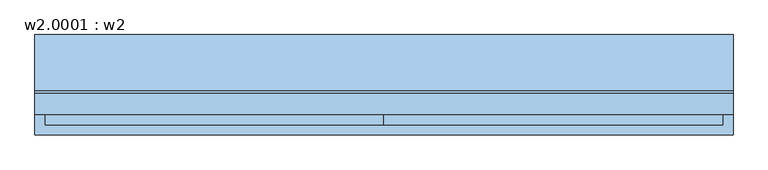
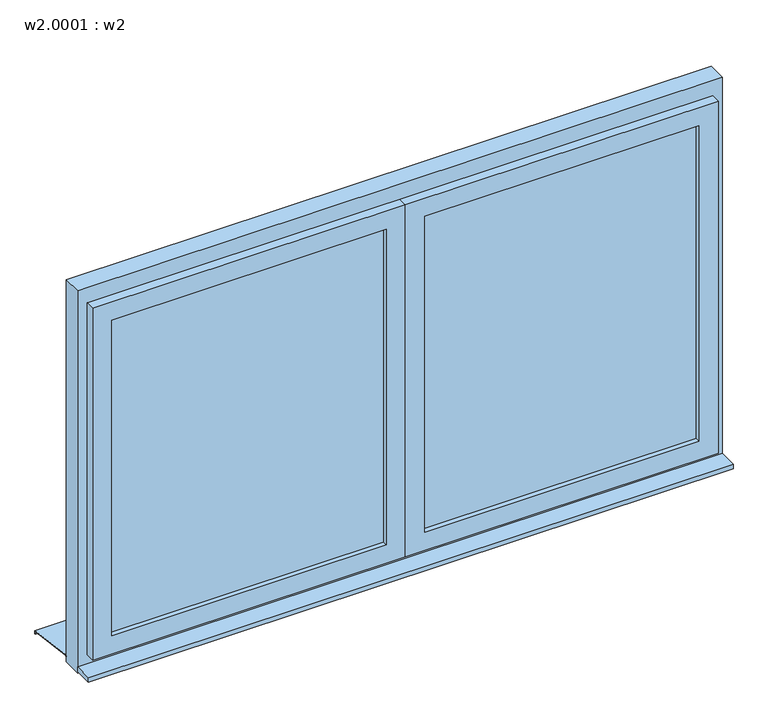
"""IFC4 building model written with IfcOpenShell, lengths in millimetres: window geometry, w2.0001 : w2."""

from ifc_helpers import new_model, si_unit, frame, origin, place, context, project, spatial, polyline, outline, extrude, faceted_brep, source, transform, mapped, element, save


def w2_0001_w2_7b90d420(model_context):
    return source(origin(), model_context, "Body", "SolidModel", [
        extrude(outline(polyline([(-15.6778457, 1020.0), (144.3, 1000.0), (144.3, 990.0), (142.3, 990.0), (142.3, 998.3604634), (-15.8759277, 1018.0), (-25.7, 1018.0), (-25.7, 1020.0), (-15.6778457, 1020.0)])), frame((-1005.0, 0.0, 0.0), z_axis=(1.0, 0.0, 0.0), x_axis=(0.0, 1.0, 0.0)), (0.0, 0.0, 1.0), 2010.0),
        extrude(outline(polyline([(-1005.0, -144.3), (-1005.0, -85.7), (1005.0, -85.7), (1005.0, -144.3), (-1005.0, -144.3)])), frame((0.0, 0.0, 1005.0), z_axis=(0.0, 0.0, 1.0), x_axis=(1.0, 0.0, 0.0)), (0.0, 0.0, 1.0), 15.0),
        extrude(outline(polyline([(60.0, -70.7), (915.0, -70.7), (915.0, -100.7), (60.0, -100.7), (60.0, -70.7)])), frame((0.0, 0.0, 1110.0), z_axis=(0.0, 0.0, 1.0), x_axis=(1.0, 0.0, 0.0)), (0.0, 0.0, 1.0), 1040.0),
        extrude(outline(polyline([(-915.0, -70.7), (-60.0, -70.7), (-60.0, -100.7), (-915.0, -100.7), (-915.0, -70.7)])), frame((0.0, 0.0, 1110.0), z_axis=(0.0, 0.0, 1.0), x_axis=(1.0, 0.0, 0.0)), (0.0, 0.0, 1.0), 1040.0),
        extrude(outline(polyline([(2260.0, -1005.0), (1000.0, -1005.0), (1000.0, 1005.0), (2260.0, 1005.0), (2260.0, -1005.0)]), holes=[polyline([(2180.0, -945.0), (2180.0, 945.0), (1080.0, 945.0), (1080.0, -945.0), (2180.0, -945.0)])]), frame((0.0, -85.7, 0.0), z_axis=(0.0, 1.0, 0.0), x_axis=(0.0, 0.0, 1.0)), (0.0, 0.0, 1.0), 60.0),
        extrude(outline(polyline([(30.0, -85.7), (-30.0, -85.7), (-30.0, -25.7), (30.0, -25.7), (30.0, -85.7)])), frame((0.0, 0.0, 1080.0), z_axis=(0.0, 0.0, 1.0), x_axis=(1.0, 0.0, 0.0)), (0.0, 0.0, 1.0), 1100.0),
        faceted_brep([(30.0, -85.7, 1080.0), (30.0, -55.7, 1080.0), (945.0, -55.7, 1080.0), (945.0, -85.7, 1080.0), (945.0, -55.7, 2180.0), (945.0, -85.7, 2180.0), (30.0, -55.7, 2180.0), (915.0, -55.7, 2150.0), (60.0, -55.7, 2150.0), (60.0, -55.7, 1110.0), (915.0, -55.7, 1110.0), (975.0, -85.7, 1050.0), (0.0, -85.7, 1050.0), (0.0, -85.7, 2210.0), (975.0, -85.7, 2210.0), (30.0, -85.7, 2180.0), (0.0, -115.7, 1050.0), (975.0, -115.7, 1050.0), (975.0, -115.7, 2210.0), (0.0, -115.7, 2210.0), (915.0, -115.7, 1110.0), (60.0, -115.7, 1110.0), (60.0, -115.7, 2150.0), (915.0, -115.7, 2150.0)], [[[0, 1, 2, 3]], [[3, 2, 4, 5]], [[2, 1, 6, 4], [7, 8, 9, 10]], [[11, 12, 13, 14], [5, 15, 0, 3]], [[16, 12, 11, 17]], [[17, 11, 14, 18]], [[18, 19, 16, 17], [20, 21, 22, 23]], [[9, 21, 20, 10]], [[10, 20, 23, 7]], [[15, 6, 1, 0]], [[19, 13, 12, 16]], [[8, 22, 21, 9]], [[5, 4, 6, 15]], [[18, 14, 13, 19]], [[7, 23, 22, 8]]]),
        faceted_brep([(-945.0, -85.7, 1080.0), (-945.0, -55.7, 1080.0), (-30.0, -55.7, 1080.0), (-30.0, -85.7, 1080.0), (-30.0, -55.7, 2180.0), (-30.0, -85.7, 2180.0), (-945.0, -55.7, 2180.0), (-60.0, -55.7, 2150.0), (-915.0, -55.7, 2150.0), (-915.0, -55.7, 1110.0), (-60.0, -55.7, 1110.0), (0.0, -85.7, 1050.0), (-975.0, -85.7, 1050.0), (-975.0, -85.7, 2210.0), (0.0, -85.7, 2210.0), (-945.0, -85.7, 2180.0), (-975.0, -115.7, 1050.0), (0.0, -115.7, 1050.0), (0.0, -115.7, 2210.0), (-975.0, -115.7, 2210.0), (-60.0, -115.7, 1110.0), (-915.0, -115.7, 1110.0), (-915.0, -115.7, 2150.0), (-60.0, -115.7, 2150.0)], [[[0, 1, 2, 3]], [[3, 2, 4, 5]], [[2, 1, 6, 4], [7, 8, 9, 10]], [[11, 12, 13, 14], [5, 15, 0, 3]], [[16, 12, 11, 17]], [[17, 11, 14, 18]], [[18, 19, 16, 17], [20, 21, 22, 23]], [[9, 21, 20, 10]], [[10, 20, 23, 7]], [[15, 6, 1, 0]], [[19, 13, 12, 16]], [[8, 22, 21, 9]], [[5, 4, 6, 15]], [[18, 14, 13, 19]], [[7, 23, 22, 8]]]),
    ])


if __name__ == "__main__":
    model = new_model("IFC4")
    model_context = context("Model", 3, world=origin())
    ifc_project = project(units=[si_unit("LENGTHUNIT", "METRE", prefix="MILLI")], contexts=[model_context])
    site = spatial("IfcSite", under=ifc_project)
    building = spatial("IfcBuilding", under=site)
    placement = place(None, origin())
    w2_0001_w2_shape = w2_0001_w2_7b90d420(model_context)
    element("IfcWindow", 1, ObjectType="w2.0001 : w2", at=placement, inside=building, context=model_context, shape_type="MappedRepresentation", body=[
        mapped(w2_0001_w2_shape, transform((0.0, 0.0, 0.0), x_axis=(1.0, 0.0, 0.0), y_axis=(0.0, 1.0, 0.0), z_axis=(0.0, 0.0, 1.0))),
    ])
    save(model, "model.ifc")

# Revit data of these elements
# Type "w2.0001 : w2"
#   Type Mark = "19"
#   Operation = "DoublePanelVertical"
#   Keynote = "16.05.01"
#   Analytic Construction = "<None>"
#   Rough Width = 6' - 7.13386"
#   Rough Height = 4' - 1.6063"
#   Rahmentiefe = 0' - 2.3622"
#   Rahmenhöhe unten = 0' - 3.14961"
#   Rahmehöhe oben = 0' - 3.14961"
#   Rahmenbreite = 0' - 2.3622"
#   Height = 4' - 1.6063"
#   Flügeltiefe = 0' - 2.3622"
#   Flügelbreite = 0' - 2.3622"
#   Einbautiefe (von außen) [instance default] = 0' - 5.51181"
#   Width = 6' - 7.13386"
#   Kippflügel [instance default] = yes
#   Drehflügel im Grundriß darstellen [instance default] = no
#   Drehflügel [instance default] = yes
#   Define Thermal Properties by = 1
#   Rahmen [instance default] = none
#   Glas [instance default] = none
#   Flügel [instance default] = none
#   Fensterbank aussen [instance default] = none
#   Fensterbank innen [instance default] = none
#   Wall Closure = (empty or 0)
# Element 1 (IfcWindow, "w2.0001 : w2")
#   Materials on its faces: "Fenster - Kunststoff", "Fenster - Kunststoff weiss", "Glass", "Fenster - Holz"
# Materials
#   "Fenster - Kunststoff": colour RGB 249 249 249, transparency 0
#   "Fenster - Kunststoff weiss": colour RGB 249 249 249, transparency 0
#   "Glass": class "Glass", colour RGB 0 128 192, transparency 0.75, Description = "Soda Lime Glass", Cost = 0
#   "Fenster - Holz": colour RGB 216 135 75, transparency 0
